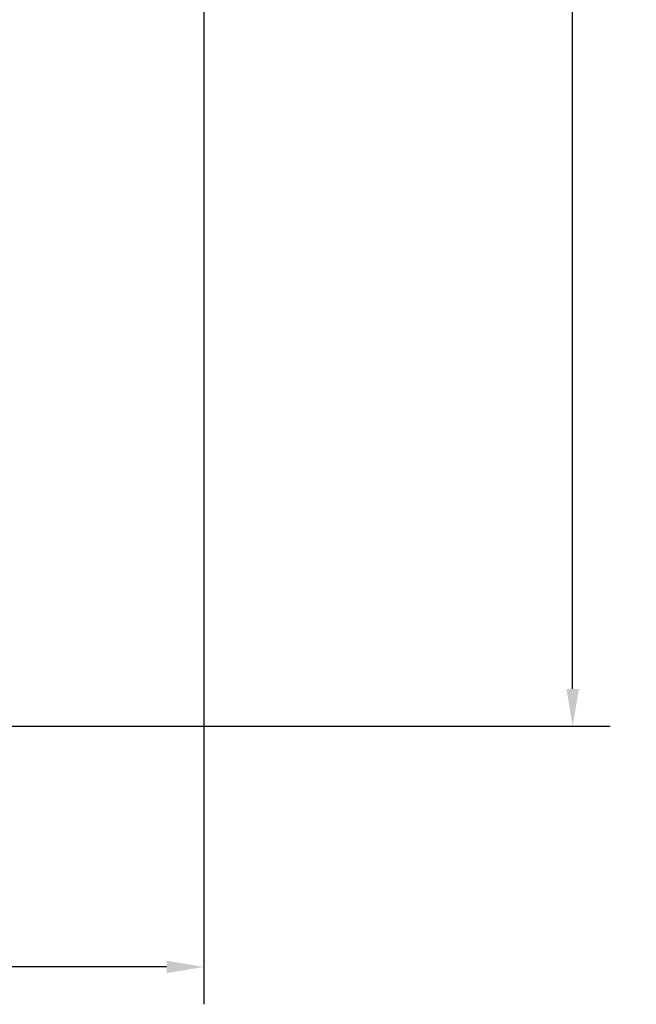
# Model space of a CAD drawing. Units: metres. Extents: x 4298.5 to 4325.2, y 2075 to 2095.8.
# Tile 26 of 35: x 4321.9 to 4324.9, y 2075 to 2079.7. Entities that reach past the tile are written whole.
import ezdxf

# ---------------------------------------------------------------- set-up
doc = ezdxf.new("R2010")
doc.units = ezdxf.units.M
doc.layers.add('A-ANNO-DIMS', color=2, linetype='Continuous', lineweight=18)
doc.styles.get("Standard").update_dxf_attribs({"font": 'arial.ttf'})
doc.dimstyles.get("Standard").update_dxf_attribs({"dimtxt": 0.18, "dimasz": 0.18, "dimexe": 0.18, "dimexo": 0.0625, "dimgap": 0.09, "dimtad": 0, "dimtih": 1, "dimtoh": 1, "dimdec": 4, "dimzin": 0, "dimdsep": 46, "dimtxsty": 'Standard', "dimcen": 0.09, "dimadec": 0, "dimazin": 0, "dimtfac": 1, "dimtdec": 4, "dimtofl": 0, "dimtmove": 0, "dimatfit": 3, "dimfxl": 1, "dimtolj": 1, "dimtzin": 0, "dimarcsym": 0})

# ---------------------------------------------------------------- blocks, each defined once
blk = doc.blocks.new('*D47')
at = {"layer": 'A-ANNO-DIMS', "color": 0, "lineweight": -2, "transparency": 16777216}
for p, q in [((4300.4306, 2084.4956), (4300.4306, 2074.9896)), ((4322.8106, 2084.4956), (4322.8106, 2074.9896)), ((4300.6106, 2075.1696), (4311.2252, 2075.1696)), ((4322.6306, 2075.1696), (4312.016, 2075.1696))]:
    blk.add_line(p, q, dxfattribs=at)
at = {"layer": 'A-ANNO-DIMS', "color": 0, "transparency": 16777216}
for points in [[(4300.6106, 2075.1996), (4300.6106, 2075.1396), (4300.4306, 2075.1696)], [(4322.6306, 2075.1996), (4322.6306, 2075.1396), (4322.8106, 2075.1696)]]:
    blk.add_solid(points, dxfattribs=at)
at = {"layer": 'Defpoints', "color": 0, "transparency": 16777216}
for p in [(4300.4306, 2084.5581), (4322.8106, 2084.5581), (4322.8106, 2075.1696)]:
    blk.add_point(p, dxfattribs=at)
at = {"layer": 'A-ANNO-DIMS', "color": 0, "transparency": 16777216, "insert": (4311.6206, 2075.1696), "char_height": 0.18, "attachment_point": 5}
blk.add_mtext('\\A1;22.38', dxfattribs=at)
blk = doc.blocks.new('*D48')
at = {"layer": 'A-ANNO-DIMS', "color": 0, "lineweight": -2, "transparency": 16777216}
for p, q in [((4310.1831, 2094.4781), (4324.7671, 2094.4781)), ((4324.5871, 2094.2981), (4324.5871, 2085.585)), ((4324.5871, 2076.5081), (4324.5871, 2085.2212)), ((4316.8731, 2076.3281), (4324.7671, 2076.3281))]:
    blk.add_line(p, q, dxfattribs=at)
at = {"layer": 'A-ANNO-DIMS', "color": 0, "transparency": 16777216}
for points in [[(4324.5571, 2094.2981), (4324.6171, 2094.2981), (4324.5871, 2094.4781)], [(4324.5571, 2076.5081), (4324.6171, 2076.5081), (4324.5871, 2076.3281)]]:
    blk.add_solid(points, dxfattribs=at)
at = {"layer": 'Defpoints', "color": 0, "transparency": 16777216}
for p in [(4310.1206, 2094.4781), (4316.8106, 2076.3281), (4324.5871, 2076.3281)]:
    blk.add_point(p, dxfattribs=at)
at = {"layer": 'A-ANNO-DIMS', "color": 0, "transparency": 16777216, "insert": (4324.5871, 2085.4031), "char_height": 0.18, "attachment_point": 5}
blk.add_mtext('\\A1;18.15', dxfattribs=at)
blk = doc.blocks.new('*D55')
at = {"layer": 'A-ANNO-DIMS', "color": 0, "lineweight": -2, "transparency": 16777216}
for p, q in [((4320.3167, 2084.4996), (4320.3167, 2074.9896)), ((4322.8106, 2084.4956), (4322.8106, 2074.9896)), ((4320.4967, 2075.1696), (4321.1688, 2075.1696)), ((4322.6306, 2075.1696), (4321.9585, 2075.1696))]:
    blk.add_line(p, q, dxfattribs=at)
at = {"layer": 'A-ANNO-DIMS', "color": 0, "transparency": 16777216}
for points in [[(4320.4967, 2075.1996), (4320.4967, 2075.1396), (4320.3167, 2075.1696)], [(4322.6306, 2075.1996), (4322.6306, 2075.1396), (4322.8106, 2075.1696)]]:
    blk.add_solid(points, dxfattribs=at)
at = {"layer": 'Defpoints', "color": 0, "transparency": 16777216}
for p in [(4320.3167, 2084.5621), (4322.8106, 2084.5581), (4322.8106, 2075.1696)]:
    blk.add_point(p, dxfattribs=at)
at = {"layer": 'A-ANNO-DIMS', "color": 0, "transparency": 16777216, "insert": (4321.5636, 2075.1696), "char_height": 0.18, "attachment_point": 5}
blk.add_mtext('\\A1;2.494', dxfattribs=at)

msp = doc.modelspace()

# ---------------------------------------------------------------- dimensions: what is measured, and where the dimension line sits
at = {"layer": 'A-ANNO-DIMS'}
dim = msp.add_linear_dim(base=(4324.5871, 2076.3281), p1=(4310.1206, 2094.4781), p2=(4316.8106, 2076.3281), angle=90, dimstyle='Standard', override={"dimdec": 2, "dimlfac": 1, "dimrnd": 0, "dimzin": 0, "dimdsep": 46, "dimlunit": 2}, dxfattribs=at)
dim.commit()
dim.dimension.update_dxf_attribs({"geometry": '*D48', "text_midpoint": (4324.5871, 2085.4031)})
for p1, override, picture, middle in [((4300.4306, 2084.5581), {"dimdec": 2, "dimlfac": 1, "dimrnd": 0, "dimzin": 0, "dimdsep": 46, "dimlunit": 2}, '*D47', (4311.6206, 2075.1696)), ((4320.3167, 2084.5621), {"dimdec": 3, "dimlfac": 1, "dimrnd": 0, "dimzin": 0, "dimdsep": 46, "dimlunit": 2}, '*D55', (4321.5636, 2075.1696))]:
    dim = msp.add_linear_dim(base=(4322.8106, 2075.1696), p1=p1, p2=(4322.8106, 2084.5581), dimstyle='Standard', override=override, dxfattribs=at)
    dim.commit()
    dim.dimension.update_dxf_attribs({"geometry": picture, "text_midpoint": middle})

doc.saveas('drawing.dxf')
